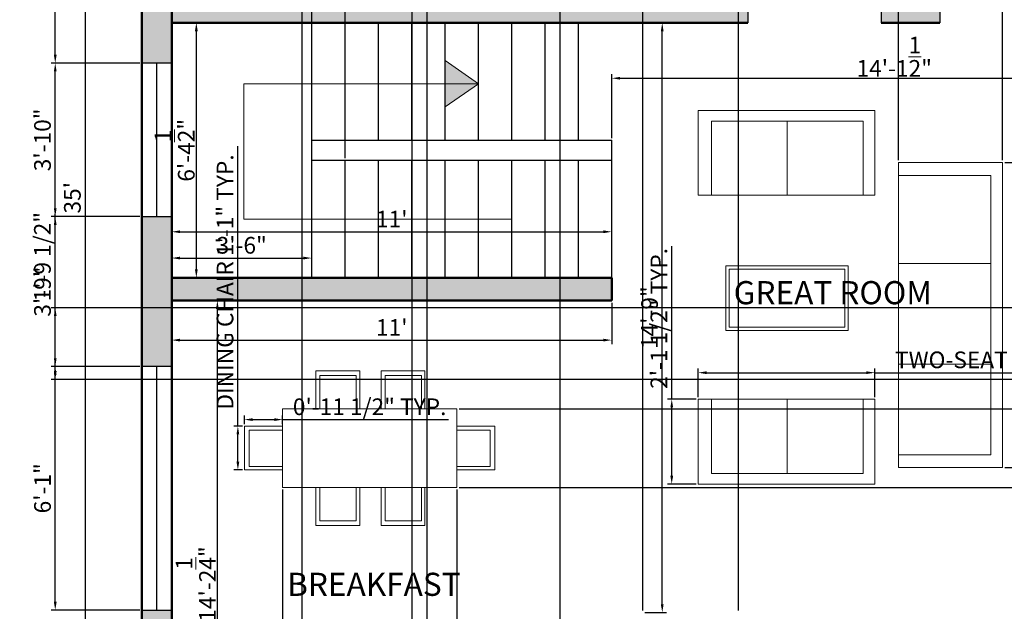
# Model space of a CAD drawing. Units: inches. Extents: x 2168 to 2706, y 2255 to 2760.
# Tile 2 of 4: x 2168 to 2463, y 2389 to 2567. Entities that reach past the tile are written whole.
import ezdxf

# ---------------------------------------------------------------- set-up
doc = ezdxf.new("R2010")
doc.units = ezdxf.units.IN
for name, color, linetype, lineweight in [('A-ANNO-DIMS', 220, 'Continuous', 18), ('A-ANNO-SYMB', 10, 'Continuous', 18), ('A-AREA-IDEN', 220, 'Continuous', 25), ('A-FLOR-STRS', 10, 'Continuous', 25), ('A-WALL-PATT', 140, 'Continuous', 13), ('DOOR', 30, 'Continuous', 25), ('FUR', 112, 'Continuous', 18), ('WALL', 140, 'Continuous', 50), ('WINDOW', 200, 'Continuous', 25)]:
    doc.layers.add(name, color=color, linetype=linetype, lineweight=lineweight)
doc.styles.get("Standard").update_dxf_attribs({"font": 'arial.ttf'})
doc.dimstyles.new('ISO-25', dxfattribs={"dimtxt": 5, "dimasz": 2.5, "dimexe": 1.25, "dimexo": 0.625, "dimtad": 1, "dimlunit": 4, "dimtxsty": 'Standard', "dimcen": 2.5, "dimadec": 0, "dimazin": 0, "dimtfac": 1, "dimtmove": 0, "dimatfit": 3, "dimfxl": 1, "dimarcsym": 0})

# ---------------------------------------------------------------- blocks, each defined once
blk = doc.blocks.new('*U2')
for p, q in [((0, 0), (0, -6)), ((40, 0), (40, -6))]:
    blk.add_line(p, q)
blk.add_lwpolyline([(0, 0), (0, 40), (1.75, 40), (1.75, 0)], close=True)
blk.add_arc((0, 0), 40, 0, 90)
blk = doc.blocks.new('*D20')
at = {"layer": 'A-ANNO-DIMS', "color": 0, "lineweight": -2, "transparency": 16777216}
for p, q in [((2213.72, 2489.97), (2213.72, 2504.39)), ((2216.22, 2503.14), (2343.22, 2503.14)), ((2345.72, 2489.97), (2345.72, 2504.39))]:
    blk.add_line(p, q, dxfattribs=at)
at = {"layer": 'A-ANNO-DIMS', "color": 0, "transparency": 16777216}
for points in [[(2216.22, 2503.56), (2216.22, 2502.73), (2213.72, 2503.14)], [(2343.22, 2503.56), (2343.22, 2502.73), (2345.72, 2503.14)]]:
    blk.add_solid(points, dxfattribs=at)
at = {"layer": 'Defpoints', "color": 0, "transparency": 16777216}
for p in [(2345.72, 2503.14), (2213.72, 2489.35), (2345.72, 2489.35)]:
    blk.add_point(p, dxfattribs=at)
at = {"layer": 'A-ANNO-DIMS', "color": 0, "transparency": 16777216, "insert": (2279.72, 2506.28), "char_height": 5, "attachment_point": 5}
blk.add_mtext("11'", dxfattribs=at)
blk = doc.blocks.new('*D21')
at = {"layer": 'A-ANNO-DIMS', "color": 0, "lineweight": -2, "transparency": 16777216}
for p, q in [((2213.72, 2489.97), (2213.72, 2496.5)), ((2255.72, 2489.97), (2255.72, 2496.5)), ((2216.22, 2495.25), (2253.22, 2495.25))]:
    blk.add_line(p, q, dxfattribs=at)
at = {"layer": 'A-ANNO-DIMS', "color": 0, "transparency": 16777216}
for points in [[(2216.22, 2495.67), (2216.22, 2494.83), (2213.72, 2495.25)], [(2253.22, 2495.67), (2253.22, 2494.83), (2255.72, 2495.25)]]:
    blk.add_solid(points, dxfattribs=at)
at = {"layer": 'Defpoints', "color": 0, "transparency": 16777216}
for p in [(2255.72, 2495.25), (2213.72, 2489.35), (2255.72, 2489.35)]:
    blk.add_point(p, dxfattribs=at)
at = {"layer": 'A-ANNO-DIMS', "color": 0, "transparency": 16777216, "insert": (2234.72, 2498.43), "char_height": 5, "attachment_point": 5}
blk.add_mtext('3\'-6"', dxfattribs=at)
blk = doc.blocks.new('*D22')
at = {"layer": 'A-ANNO-DIMS', "color": 0, "lineweight": -2, "transparency": 16777216}
for p, q in [((2214.35, 2565.85), (2222.35, 2565.85)), ((2221.1, 2491.85), (2221.1, 2563.35)), ((2214.35, 2489.35), (2222.35, 2489.35))]:
    blk.add_line(p, q, dxfattribs=at)
at = {"layer": 'A-ANNO-DIMS', "color": 0, "transparency": 16777216}
for points in [[(2220.68, 2563.35), (2221.52, 2563.35), (2221.1, 2565.85)], [(2220.68, 2491.85), (2221.52, 2491.85), (2221.1, 2489.35)]]:
    blk.add_solid(points, dxfattribs=at)
at = {"layer": 'Defpoints', "color": 0, "transparency": 16777216}
for p in [(2213.72, 2565.85), (2221.1, 2565.85), (2213.72, 2489.35)]:
    blk.add_point(p, dxfattribs=at)
at = {"layer": 'A-ANNO-DIMS', "color": 0, "transparency": 16777216, "insert": (2214.58, 2527.6), "char_height": 5, "attachment_point": 5, "rotation": 90}
blk.add_mtext('6\'-4{\\H1x;\\S1/2;}"', dxfattribs=at)
blk = doc.blocks.new('*D23')
at = {"layer": 'A-ANNO-DIMS', "color": 0, "lineweight": -2, "transparency": 16777216}
for p, q in [((2345.72, 2531.22), (2345.72, 2550.47)), ((2348.22, 2549.22), (2512.72, 2549.22)), ((2515.22, 2531.22), (2515.22, 2550.47))]:
    blk.add_line(p, q, dxfattribs=at)
at = {"layer": 'A-ANNO-DIMS', "color": 0, "transparency": 16777216}
for points in [[(2348.22, 2549.63), (2348.22, 2548.8), (2345.72, 2549.22)], [(2512.72, 2549.63), (2512.72, 2548.8), (2515.22, 2549.22)]]:
    blk.add_solid(points, dxfattribs=at)
at = {"layer": 'Defpoints', "color": 0, "transparency": 16777216}
for p in [(2515.22, 2549.22), (2345.72, 2530.6), (2515.22, 2530.6)]:
    blk.add_point(p, dxfattribs=at)
at = {"layer": 'A-ANNO-DIMS', "color": 0, "transparency": 16777216, "insert": (2430.47, 2555.69), "char_height": 5, "attachment_point": 5}
blk.add_mtext('14\'-1{\\H1x;\\S1/2;}"', dxfattribs=at)
blk = doc.blocks.new('*D24')
at = {"layer": 'A-ANNO-DIMS', "color": 0, "lineweight": -2, "transparency": 16777216}
for p, q in [((2355.67, 2565.85), (2362.12, 2565.85)), ((2360.87, 2391.35), (2360.87, 2563.35)), ((2355.67, 2388.85), (2362.12, 2388.85))]:
    blk.add_line(p, q, dxfattribs=at)
at = {"layer": 'A-ANNO-DIMS', "color": 0, "transparency": 16777216}
for points in [[(2360.45, 2563.35), (2361.28, 2563.35), (2360.87, 2565.85)], [(2360.45, 2391.35), (2361.28, 2391.35), (2360.87, 2388.85)]]:
    blk.add_solid(points, dxfattribs=at)
at = {"layer": 'Defpoints', "color": 0, "transparency": 16777216}
for p in [(2355.04, 2565.85), (2360.87, 2565.85), (2355.04, 2388.85)]:
    blk.add_point(p, dxfattribs=at)
at = {"layer": 'A-ANNO-DIMS', "color": 0, "transparency": 16777216, "insert": (2357.69, 2477.35), "char_height": 5, "attachment_point": 5, "rotation": 90}
blk.add_mtext('14\'-9"', dxfattribs=at)
blk = doc.blocks.new('*D25')
at = {"layer": 'A-ANNO-DIMS', "color": 0, "lineweight": -2, "transparency": 16777216}
for p, q in [((2213.72, 2481.86), (2213.72, 2469.37)), ((2345.72, 2481.86), (2345.72, 2469.37)), ((2216.22, 2470.62), (2343.22, 2470.62))]:
    blk.add_line(p, q, dxfattribs=at)
at = {"layer": 'A-ANNO-DIMS', "color": 0, "transparency": 16777216}
for points in [[(2216.22, 2471.04), (2216.22, 2470.21), (2213.72, 2470.62)], [(2343.22, 2471.04), (2343.22, 2470.21), (2345.72, 2470.62)]]:
    blk.add_solid(points, dxfattribs=at)
at = {"layer": 'Defpoints', "color": 0, "transparency": 16777216}
for p in [(2213.72, 2482.49), (2345.72, 2482.49), (2345.72, 2470.62)]:
    blk.add_point(p, dxfattribs=at)
at = {"layer": 'A-ANNO-DIMS', "color": 0, "transparency": 16777216, "insert": (2279.72, 2473.76), "char_height": 5, "attachment_point": 5}
blk.add_mtext("11'", dxfattribs=at)
blk = doc.blocks.new('*D28')
at = {"layer": 'A-ANNO-DIMS', "color": 0, "lineweight": -2, "transparency": 16777216}
for p, q in [((2214.35, 2482.49), (2228.66, 2482.49)), ((2227.41, 2314.85), (2227.41, 2479.99)), ((2214.35, 2312.35), (2228.66, 2312.35))]:
    blk.add_line(p, q, dxfattribs=at)
at = {"layer": 'A-ANNO-DIMS', "color": 0, "transparency": 16777216}
for points in [[(2227, 2479.99), (2227.83, 2479.99), (2227.41, 2482.49)], [(2227, 2314.85), (2227.83, 2314.85), (2227.41, 2312.35)]]:
    blk.add_solid(points, dxfattribs=at)
at = {"layer": 'Defpoints', "color": 0, "transparency": 16777216}
for p in [(2213.72, 2482.49), (2227.41, 2482.49), (2213.72, 2312.35)]:
    blk.add_point(p, dxfattribs=at)
at = {"layer": 'A-ANNO-DIMS', "color": 0, "transparency": 16777216, "insert": (2220.94, 2397.42), "char_height": 5, "attachment_point": 5, "rotation": 90}
blk.add_mtext('14\'-2{\\H1x;\\S1/4;}"', dxfattribs=at)
blk = doc.blocks.new('*D30')
at = {"layer": 'A-ANNO-DIMS', "color": 0, "lineweight": -2, "transparency": 16777216}
for p, q in [((2204.1, 2723.35), (2186.49, 2723.35)), ((2187.74, 2720.85), (2187.74, 2305.85)), ((2204.1, 2303.35), (2186.49, 2303.35))]:
    blk.add_line(p, q, dxfattribs=at)
at = {"layer": 'A-ANNO-DIMS', "color": 0, "transparency": 16777216}
for points in [[(2187.33, 2720.85), (2188.16, 2720.85), (2187.74, 2723.35)], [(2187.33, 2305.85), (2188.16, 2305.85), (2187.74, 2303.35)]]:
    blk.add_solid(points, dxfattribs=at)
at = {"layer": 'Defpoints', "color": 0, "transparency": 16777216}
for p in [(2204.72, 2723.35), (2187.74, 2303.35), (2204.72, 2303.35)]:
    blk.add_point(p, dxfattribs=at)
at = {"layer": 'A-ANNO-DIMS', "color": 0, "transparency": 16777216, "insert": (2184.56, 2513.35), "char_height": 5, "attachment_point": 5, "rotation": 90}
blk.add_mtext("35'", dxfattribs=at)
blk = doc.blocks.new('CHAIR-DINING')
for p, q in [((-11.42, -6.49), (-11.42, 6.66)), ((-11.42, 6.66), (0, 6.66)), ((0, -6.49), (-11.42, -6.49))]:
    blk.add_line(p, q)
blk.add_lwpolyline([(0, 5.44), (-10.02, 5.44), (-10.02, -5.44), (0, -5.44)], close=True)
blk = doc.blocks.new('SOFA-TWO-SEAT')
for p, q in [((3.96, 25.48), (0, 25.48)), ((0, 25.48), (0, 0)), ((26.73, 25.48), (26.73, 3.2)), ((52.95, 25.48), (48.19, 25.48)), ((52.95, 0), (52.95, 25.48)), ((0, 0), (52.95, 0))]:
    blk.add_line(p, q)
blk.add_lwpolyline([(49.5, 3.2), (3.96, 3.2), (3.96, 25.48), (49.5, 25.48)], close=True)
blk = doc.blocks.new('*D38')
at = {"layer": 'A-ANNO-DIMS', "color": 0, "lineweight": -2, "transparency": 16777216}
for p, q in [((2233.56, 2444.79), (2233.56, 2528.83)), ((2234.91, 2444.79), (2232.31, 2444.79)), ((2233.56, 2434.14), (2233.56, 2442.29)), ((2234.91, 2431.64), (2232.31, 2431.64))]:
    blk.add_line(p, q, dxfattribs=at)
at = {"layer": 'A-ANNO-DIMS', "color": 0, "transparency": 16777216}
for points in [[(2233.14, 2442.29), (2233.98, 2442.29), (2233.56, 2444.79)], [(2233.14, 2434.14), (2233.98, 2434.14), (2233.56, 2431.64)]]:
    blk.add_solid(points, dxfattribs=at)
at = {"layer": 'Defpoints', "color": 0, "transparency": 16777216}
for p in [(2233.56, 2444.79), (2235.53, 2444.79), (2235.53, 2431.64)]:
    blk.add_point(p, dxfattribs=at)
at = {"layer": 'A-ANNO-DIMS', "color": 0, "transparency": 16777216, "insert": (2230.35, 2488.06), "char_height": 5, "attachment_point": 5, "rotation": 90}
blk.add_mtext('DINING CHAIR 1\'-1" TYP.', dxfattribs=at)
blk = doc.blocks.new('*D39')
at = {"layer": 'A-ANNO-DIMS', "color": 0, "lineweight": -2, "transparency": 16777216}
for p, q in [((2235.53, 2445.41), (2235.53, 2448.01)), ((2238.03, 2446.76), (2244.46, 2446.76)), ((2246.96, 2445.41), (2246.96, 2448.01)), ((2246.96, 2446.76), (2296.72, 2446.76))]:
    blk.add_line(p, q, dxfattribs=at)
at = {"layer": 'A-ANNO-DIMS', "color": 0, "transparency": 16777216}
for points in [[(2238.03, 2447.18), (2238.03, 2446.34), (2235.53, 2446.76)], [(2244.46, 2447.18), (2244.46, 2446.34), (2246.96, 2446.76)]]:
    blk.add_solid(points, dxfattribs=at)
at = {"layer": 'Defpoints', "color": 0, "transparency": 16777216}
for p in [(2246.96, 2446.76), (2235.53, 2444.79), (2246.96, 2444.79)]:
    blk.add_point(p, dxfattribs=at)
at = {"layer": 'A-ANNO-DIMS', "color": 0, "transparency": 16777216, "insert": (2273.09, 2449.97), "char_height": 5, "attachment_point": 5}
blk.add_mtext('0\'-11 1/2" TYP.', dxfattribs=at)
blk = doc.blocks.new('*D40')
at = {"layer": 'A-ANNO-DIMS', "color": 0, "lineweight": -2, "transparency": 16777216}
for p, q in [((2371.67, 2453.52), (2371.67, 2462.09)), ((2374.17, 2460.84), (2422.11, 2460.84)), ((2424.61, 2453.52), (2424.61, 2462.09)), ((2424.61, 2460.84), (2518.73, 2460.84))]:
    blk.add_line(p, q, dxfattribs=at)
at = {"layer": 'A-ANNO-DIMS', "color": 0, "transparency": 16777216}
for points in [[(2374.17, 2461.26), (2374.17, 2460.43), (2371.67, 2460.84)], [(2422.11, 2461.26), (2422.11, 2460.43), (2424.61, 2460.84)]]:
    blk.add_solid(points, dxfattribs=at)
at = {"layer": 'Defpoints', "color": 0, "transparency": 16777216}
for p in [(2424.61, 2460.84), (2371.67, 2452.9), (2424.61, 2452.9)]:
    blk.add_point(p, dxfattribs=at)
at = {"layer": 'A-ANNO-DIMS', "color": 0, "transparency": 16777216, "insert": (2472.92, 2464.05), "char_height": 5, "attachment_point": 5}
blk.add_mtext('TWO-SEAT SOFA 4\'-5" TYP.', dxfattribs=at)
blk = doc.blocks.new('*D41')
at = {"layer": 'A-ANNO-DIMS', "color": 0, "lineweight": -2, "transparency": 16777216}
for p, q in [((2363.72, 2452.9), (2363.72, 2498.86)), ((2371.04, 2452.9), (2362.47, 2452.9)), ((2363.72, 2429.92), (2363.72, 2450.4)), ((2371.04, 2427.42), (2362.47, 2427.42))]:
    blk.add_line(p, q, dxfattribs=at)
at = {"layer": 'A-ANNO-DIMS', "color": 0, "transparency": 16777216}
for points in [[(2363.31, 2450.4), (2364.14, 2450.4), (2363.72, 2452.9)], [(2363.31, 2429.92), (2364.14, 2429.92), (2363.72, 2427.42)]]:
    blk.add_solid(points, dxfattribs=at)
at = {"layer": 'Defpoints', "color": 0, "transparency": 16777216}
for p in [(2363.72, 2452.9), (2371.67, 2452.9), (2371.67, 2427.42)]:
    blk.add_point(p, dxfattribs=at)
at = {"layer": 'A-ANNO-DIMS', "color": 0, "transparency": 16777216, "insert": (2360.51, 2477.13), "char_height": 5, "attachment_point": 5, "rotation": 90}
blk.add_mtext('2\'-1 1/2" TYP.', dxfattribs=at)
blk = doc.blocks.new('*D49')
at = {"layer": 'A-ANNO-DIMS', "color": 0, "lineweight": -2, "transparency": 16777216}
for p, q in [((2355.04, 2389.47), (2355.04, 2750.55)), ((2383.78, 2389.47), (2383.78, 2750.55)), ((2357.54, 2749.3), (2381.28, 2749.3))]:
    blk.add_line(p, q, dxfattribs=at)
at = {"layer": 'A-ANNO-DIMS', "color": 0, "transparency": 16777216}
for points in [[(2357.54, 2749.71), (2357.54, 2748.88), (2355.04, 2749.3)], [(2381.28, 2749.71), (2381.28, 2748.88), (2383.78, 2749.3)]]:
    blk.add_solid(points, dxfattribs=at)
at = {"layer": 'Defpoints', "color": 0, "transparency": 16777216}
for p in [(2383.78, 2749.3), (2355.04, 2388.85), (2383.78, 2388.85)]:
    blk.add_point(p, dxfattribs=at)
at = {"layer": 'A-ANNO-DIMS', "color": 0, "transparency": 16777216, "insert": (2369.41, 2752.51), "char_height": 5, "attachment_point": 5}
blk.add_mtext('2\'-4 1/2"', dxfattribs=at)
blk = doc.blocks.new('*D51')
at = {"layer": 'A-ANNO-DIMS', "color": 0, "lineweight": -2, "transparency": 16777216}
for p, q in [((2178.77, 2480.31), (2178.77, 2508.53)), ((2538.6, 2480.31), (2177.52, 2480.31)), ((2178.77, 2461.31), (2178.77, 2477.81)), ((2538.6, 2458.81), (2177.52, 2458.81))]:
    blk.add_line(p, q, dxfattribs=at)
at = {"layer": 'A-ANNO-DIMS', "color": 0, "transparency": 16777216}
for points in [[(2178.36, 2477.81), (2179.19, 2477.81), (2178.77, 2480.31)], [(2178.36, 2461.31), (2179.19, 2461.31), (2178.77, 2458.81)]]:
    blk.add_solid(points, dxfattribs=at)
at = {"layer": 'Defpoints', "color": 0, "transparency": 16777216}
for p in [(2178.77, 2480.31), (2539.22, 2480.31), (2539.22, 2458.81)]:
    blk.add_point(p, dxfattribs=at)
at = {"layer": 'A-ANNO-DIMS', "color": 0, "transparency": 16777216, "insert": (2175.56, 2495.67), "char_height": 5, "attachment_point": 5, "rotation": 90}
blk.add_mtext('1\'-9 1/2"', dxfattribs=at)
blk = doc.blocks.new('*D52')
at = {"layer": 'A-ANNO-DIMS', "color": 0, "lineweight": -2, "transparency": 16777216}
for p, q in [((2463.6, 2523.98), (2702.92, 2523.98)), ((2701.67, 2434.92), (2701.67, 2521.48)), ((2463.6, 2432.42), (2702.92, 2432.42))]:
    blk.add_line(p, q, dxfattribs=at)
at = {"layer": 'A-ANNO-DIMS', "color": 0, "transparency": 16777216}
for points in [[(2701.26, 2521.48), (2702.09, 2521.48), (2701.67, 2523.98)], [(2701.26, 2434.92), (2702.09, 2434.92), (2701.67, 2432.42)]]:
    blk.add_solid(points, dxfattribs=at)
at = {"layer": 'Defpoints', "color": 0, "transparency": 16777216}
for p in [(2462.98, 2523.98), (2701.67, 2523.98), (2462.98, 2432.42)]:
    blk.add_point(p, dxfattribs=at)
at = {"layer": 'A-ANNO-DIMS', "color": 0, "transparency": 16777216, "insert": (2698.46, 2478.2), "char_height": 5, "attachment_point": 5, "rotation": 90}
blk.add_mtext('7\'-7 1/2"', dxfattribs=at)
blk = doc.blocks.new('*D53')
at = {"layer": 'A-ANNO-DIMS', "color": 0, "lineweight": -2, "transparency": 16777216}
for p, q in [((2431.71, 2524.6), (2431.71, 2750.55)), ((2462.98, 2524.6), (2462.98, 2750.55)), ((2434.21, 2749.3), (2460.48, 2749.3))]:
    blk.add_line(p, q, dxfattribs=at)
at = {"layer": 'A-ANNO-DIMS', "color": 0, "transparency": 16777216}
for points in [[(2434.21, 2749.71), (2434.21, 2748.88), (2431.71, 2749.3)], [(2460.48, 2749.71), (2460.48, 2748.88), (2462.98, 2749.3)]]:
    blk.add_solid(points, dxfattribs=at)
at = {"layer": 'Defpoints', "color": 0, "transparency": 16777216}
for p in [(2462.98, 2749.3), (2431.71, 2523.98), (2462.98, 2523.98)]:
    blk.add_point(p, dxfattribs=at)
at = {"layer": 'A-ANNO-DIMS', "color": 0, "transparency": 16777216, "insert": (2447.34, 2752.51), "char_height": 5, "attachment_point": 5}
blk.add_mtext('2\'-7 1/2"', dxfattribs=at)
blk = doc.blocks.new('*D54')
at = {"layer": 'A-ANNO-DIMS', "color": 0, "lineweight": -2, "transparency": 16777216}
for p, q in [((2246.96, 2425.79), (2246.96, 2276.15)), ((2299.27, 2425.79), (2299.27, 2276.15)), ((2249.46, 2277.4), (2296.77, 2277.4))]:
    blk.add_line(p, q, dxfattribs=at)
at = {"layer": 'A-ANNO-DIMS', "color": 0, "transparency": 16777216}
for points in [[(2249.46, 2277.81), (2249.46, 2276.98), (2246.96, 2277.4)], [(2296.77, 2277.81), (2296.77, 2276.98), (2299.27, 2277.4)]]:
    blk.add_solid(points, dxfattribs=at)
at = {"layer": 'Defpoints', "color": 0, "transparency": 16777216}
for p in [(2246.96, 2426.42), (2299.27, 2426.42), (2299.27, 2277.4)]:
    blk.add_point(p, dxfattribs=at)
at = {"layer": 'A-ANNO-DIMS', "color": 0, "transparency": 16777216, "insert": (2273.11, 2280.61), "char_height": 5, "attachment_point": 5}
blk.add_mtext('4\'-4 1/2"', dxfattribs=at)
blk = doc.blocks.new('*D55')
at = {"layer": 'A-ANNO-DIMS', "color": 0, "lineweight": -2, "transparency": 16777216}
for p, q in [((2299.9, 2450), (2702.92, 2450)), ((2701.67, 2447.5), (2701.67, 2428.92)), ((2299.9, 2426.42), (2702.92, 2426.42)), ((2701.67, 2426.42), (2701.67, 2394.31))]:
    blk.add_line(p, q, dxfattribs=at)
at = {"layer": 'A-ANNO-DIMS', "color": 0, "transparency": 16777216}
for points in [[(2701.26, 2447.5), (2702.09, 2447.5), (2701.67, 2450)], [(2701.26, 2428.92), (2702.09, 2428.92), (2701.67, 2426.42)]]:
    blk.add_solid(points, dxfattribs=at)
at = {"layer": 'Defpoints', "color": 0, "transparency": 16777216}
for p in [(2299.27, 2450), (2299.27, 2426.42), (2701.67, 2426.42)]:
    blk.add_point(p, dxfattribs=at)
at = {"layer": 'A-ANNO-DIMS', "color": 0, "transparency": 16777216, "insert": (2698.46, 2409.11), "char_height": 5, "attachment_point": 5, "rotation": 90}
blk.add_mtext('1\'-11 1/2"', dxfattribs=at)
blk = doc.blocks.new('*D64')
at = {"layer": 'A-ANNO-DIMS', "color": 0, "lineweight": -2, "transparency": 16777216}
for p, q in [((2290.22, 2713.72), (2290.22, 2276.15)), ((2330.12, 2713.72), (2330.12, 2276.15)), ((2292.72, 2277.4), (2327.62, 2277.4))]:
    blk.add_line(p, q, dxfattribs=at)
at = {"layer": 'A-ANNO-DIMS', "color": 0, "transparency": 16777216}
for points in [[(2292.72, 2277.81), (2292.72, 2276.98), (2290.22, 2277.4)], [(2327.62, 2277.81), (2327.62, 2276.98), (2330.12, 2277.4)]]:
    blk.add_solid(points, dxfattribs=at)
at = {"layer": 'Defpoints', "color": 0, "transparency": 16777216}
for p in [(2290.22, 2714.35), (2330.12, 2714.35), (2330.12, 2277.4)]:
    blk.add_point(p, dxfattribs=at)
at = {"layer": 'A-ANNO-DIMS', "color": 0, "transparency": 16777216, "insert": (2310.17, 2280.58), "char_height": 5, "attachment_point": 5}
blk.add_mtext('3\'-4"', dxfattribs=at)
blk = doc.blocks.new('*D66')
at = {"layer": 'A-ANNO-DIMS', "color": 0, "lineweight": -2, "transparency": 16777216}
for p, q in [((2204.1, 2462.7), (2177.52, 2462.7)), ((2178.77, 2392.09), (2178.77, 2460.2)), ((2204.1, 2389.59), (2177.52, 2389.59))]:
    blk.add_line(p, q, dxfattribs=at)
at = {"layer": 'A-ANNO-DIMS', "color": 0, "transparency": 16777216}
for points in [[(2178.36, 2460.2), (2179.19, 2460.2), (2178.77, 2462.7)], [(2178.36, 2392.09), (2179.19, 2392.09), (2178.77, 2389.59)]]:
    blk.add_solid(points, dxfattribs=at)
at = {"layer": 'Defpoints', "color": 0, "transparency": 16777216}
for p in [(2178.77, 2462.7), (2204.72, 2462.7), (2204.72, 2389.59)]:
    blk.add_point(p, dxfattribs=at)
at = {"layer": 'A-ANNO-DIMS', "color": 0, "transparency": 16777216, "insert": (2175.6, 2426.14), "char_height": 5, "attachment_point": 5, "rotation": 90}
blk.add_mtext('6\'-1"', dxfattribs=at)
blk = doc.blocks.new('*D67')
at = {"layer": 'A-ANNO-DIMS', "color": 0, "lineweight": -2, "transparency": 16777216}
for p, q in [((2204.1, 2553.76), (2177.52, 2553.76)), ((2178.77, 2510.18), (2178.77, 2551.26)), ((2204.1, 2507.68), (2177.52, 2507.68))]:
    blk.add_line(p, q, dxfattribs=at)
at = {"layer": 'A-ANNO-DIMS', "color": 0, "transparency": 16777216}
for points in [[(2178.36, 2551.26), (2179.19, 2551.26), (2178.77, 2553.76)], [(2178.36, 2510.18), (2179.19, 2510.18), (2178.77, 2507.68)]]:
    blk.add_solid(points, dxfattribs=at)
at = {"layer": 'Defpoints', "color": 0, "transparency": 16777216}
for p in [(2178.77, 2553.76), (2204.72, 2553.76), (2204.72, 2507.68)]:
    blk.add_point(p, dxfattribs=at)
at = {"layer": 'A-ANNO-DIMS', "color": 0, "transparency": 16777216, "insert": (2175.59, 2530.72), "char_height": 5, "attachment_point": 5, "rotation": 90}
blk.add_mtext('3\'-10"', dxfattribs=at)
blk = doc.blocks.new('*D70')
at = {"layer": 'A-ANNO-DIMS', "color": 0, "lineweight": -2, "transparency": 16777216}
for p, q in [((2204.1, 2507.68), (2177.52, 2507.68)), ((2178.77, 2465.2), (2178.77, 2505.18)), ((2204.1, 2462.7), (2177.52, 2462.7))]:
    blk.add_line(p, q, dxfattribs=at)
at = {"layer": 'A-ANNO-DIMS', "color": 0, "transparency": 16777216}
for points in [[(2178.36, 2505.18), (2179.19, 2505.18), (2178.77, 2507.68)], [(2178.36, 2465.2), (2179.19, 2465.2), (2178.77, 2462.7)]]:
    blk.add_solid(points, dxfattribs=at)
at = {"layer": 'Defpoints', "color": 0, "transparency": 16777216}
for p in [(2178.77, 2507.68), (2204.72, 2507.68), (2204.72, 2462.7)]:
    blk.add_point(p, dxfattribs=at)
at = {"layer": 'A-ANNO-DIMS', "color": 0, "transparency": 16777216, "insert": (2175.59, 2485.19), "char_height": 5, "attachment_point": 5, "rotation": 90}
blk.add_mtext('3\'-9"', dxfattribs=at)
blk = doc.blocks.new('*D71')
at = {"layer": 'A-ANNO-DIMS', "color": 0, "lineweight": -2, "transparency": 16777216}
for p, q in [((2204.1, 2613.73), (2177.52, 2613.73)), ((2178.77, 2556.26), (2178.77, 2611.23)), ((2204.1, 2553.76), (2177.52, 2553.76))]:
    blk.add_line(p, q, dxfattribs=at)
at = {"layer": 'A-ANNO-DIMS', "color": 0, "transparency": 16777216}
for points in [[(2178.36, 2611.23), (2179.19, 2611.23), (2178.77, 2613.73)], [(2178.36, 2556.26), (2179.19, 2556.26), (2178.77, 2553.76)]]:
    blk.add_solid(points, dxfattribs=at)
at = {"layer": 'Defpoints', "color": 0, "transparency": 16777216}
for p in [(2178.77, 2613.73), (2204.72, 2613.73), (2204.72, 2553.76)]:
    blk.add_point(p, dxfattribs=at)
at = {"layer": 'A-ANNO-DIMS', "color": 0, "transparency": 16777216, "insert": (2175.6, 2583.75), "char_height": 5, "attachment_point": 5, "rotation": 90}
blk.add_mtext('5\'-0"', dxfattribs=at)
blk = doc.blocks.new('*D74')
at = {"layer": 'A-ANNO-DIMS', "color": 0, "lineweight": -2, "transparency": 16777216}
for p, q in [((2255.72, 2525.22), (2255.72, 2750.55)), ((2265.72, 2525.22), (2265.72, 2750.55)), ((2258.22, 2749.3), (2263.22, 2749.3)), ((2265.72, 2749.3), (2286.65, 2749.3))]:
    blk.add_line(p, q, dxfattribs=at)
at = {"layer": 'A-ANNO-DIMS', "color": 0, "transparency": 16777216}
for points in [[(2258.22, 2749.71), (2258.22, 2748.88), (2255.72, 2749.3)], [(2263.22, 2749.71), (2263.22, 2748.88), (2265.72, 2749.3)]]:
    blk.add_solid(points, dxfattribs=at)
at = {"layer": 'Defpoints', "color": 0, "transparency": 16777216}
for p in [(2265.72, 2749.3), (2255.72, 2524.6), (2265.72, 2524.6)]:
    blk.add_point(p, dxfattribs=at)
at = {"layer": 'A-ANNO-DIMS', "color": 0, "transparency": 16777216, "insert": (2277.44, 2752.47), "char_height": 5, "attachment_point": 5}
blk.add_mtext('0\'-10"', dxfattribs=at)
blk = doc.blocks.new('*D76')
at = {"layer": 'A-ANNO-DIMS', "color": 0, "lineweight": -2, "transparency": 16777216}
for p, q in [((2252.72, 2623.46), (2252.72, 2276.15)), ((2285.72, 2612.95), (2285.72, 2276.15)), ((2255.22, 2277.4), (2283.22, 2277.4))]:
    blk.add_line(p, q, dxfattribs=at)
at = {"layer": 'A-ANNO-DIMS', "color": 0, "transparency": 16777216}
for points in [[(2255.22, 2277.81), (2255.22, 2276.98), (2252.72, 2277.4)], [(2283.22, 2277.81), (2283.22, 2276.98), (2285.72, 2277.4)]]:
    blk.add_solid(points, dxfattribs=at)
at = {"layer": 'Defpoints', "color": 0, "transparency": 16777216}
for p in [(2252.72, 2624.08), (2285.72, 2613.58), (2285.72, 2277.4)]:
    blk.add_point(p, dxfattribs=at)
at = {"layer": 'A-ANNO-DIMS', "color": 0, "transparency": 16777216, "insert": (2269.22, 2280.57), "char_height": 5, "attachment_point": 5}
blk.add_mtext('2\'-9"', dxfattribs=at)

msp = doc.modelspace()

# ---------------------------------------------------------------- hatches: boundary and pattern name
at = {"layer": 'A-ANNO-SYMB'}
h = msp.add_hatch(color=256, dxfattribs=at)
h.dxf.hatch_style = 1
h.paths.add_polyline_path([(2305.724, 2547.588), (2295.724, 2547.588), (2295.724, 2540.636)])
h.paths.add_polyline_path([(2295.724, 2554.541), (2295.724, 2547.588), (2305.724, 2547.588)])
at = {"layer": 'A-WALL-PATT'}
h = msp.add_hatch(color=256, dxfattribs=at)
h.dxf.hatch_style = 1
h.paths.add_polyline_path([(2330.12, 2723.347), (2204.724, 2723.347), (2204.724, 2662.147), (2213.724, 2662.147), (2213.724, 2714.347), (2285.724, 2714.347), (2330.12, 2714.347)])
h.paths.add_polyline_path([(2496.542, 2723.347), (2396.128, 2723.347), (2396.128, 2714.347), (2434.224, 2714.347), (2496.542, 2714.347)])
h.paths.add_polyline_path([(2624.724, 2723.347), (2562.55, 2723.347), (2562.55, 2714.347), (2615.724, 2714.347), (2615.724, 2545.448), (2624.724, 2545.448)])
h.paths.add_polyline_path([(2438.724, 2714.347), (2434.224, 2714.347), (2434.224, 2570.347), (2426.591, 2570.347), (2426.591, 2565.847), (2438.724, 2565.847), (2444.149, 2565.847), (2444.149, 2570.347), (2438.724, 2570.347)])
h.paths.add_polyline_path([(2290.224, 2668.023), (2285.724, 2668.023), (2285.724, 2570.347), (2213.724, 2570.347), (2213.724, 2565.847), (2290.224, 2565.847), (2386.591, 2565.847), (2386.591, 2570.347), (2290.224, 2570.347)])
h.paths.add_polyline_path([(2514.678, 2570.347), (2514.678, 2630.11), (2560.439, 2630.11), (2560.439, 2570.347)], flags=16)
h.paths.add_polyline_path([(2517.528, 2574.595), (2517.528, 2583.399), (2536.063, 2583.399), (2536.063, 2574.595)], flags=0)
h.paths.add_polyline_path([(2523.909, 2586.89), (2514.678, 2597.212), (2518.822, 2600.918)], flags=0)
h.paths.add_polyline_path([(2538.189, 2574.595), (2538.189, 2583.399), (2556.724, 2583.399), (2556.724, 2574.595)], flags=0)
h.paths.add_polyline_path([(2560.439, 2630.11), (2560.439, 2570.347), (2514.678, 2570.347), (2514.678, 2630.11)])
h.paths.add_polyline_path([(2213.724, 2389.588), (2204.724, 2389.588), (2204.724, 2303.347), (2229.06, 2303.347), (2229.06, 2312.347), (2213.724, 2312.347)])
h.paths.add_polyline_path([(2213.724, 2507.677), (2204.724, 2507.677), (2204.724, 2462.696), (2213.724, 2462.696)])
h.paths.add_polyline_path([(2204.724, 2553.759), (2213.724, 2553.759), (2213.724, 2613.731), (2204.724, 2613.731)])
h = msp.add_hatch(color=256, dxfattribs=at)
h.dxf.hatch_style = 1
h.paths.add_polyline_path([(2345.724, 2489.347), (2213.724, 2489.347), (2213.724, 2482.487), (2345.724, 2482.487)])

# ---------------------------------------------------------------- linework, layer by layer
at = {"layer": 'A-ANNO-SYMB'}
for p, q in [((2305.724, 2547.588), (2295.724, 2554.541)), ((2235.327, 2506.972), (2235.327, 2547.588)), ((2235.327, 2547.588), (2305.724, 2547.588)), ((2305.724, 2547.588), (2295.724, 2540.636)), ((2315.724, 2506.972), (2235.327, 2506.972))]:
    msp.add_line(p, q, dxfattribs=at)
at = {"layer": 'A-FLOR-STRS'}
for p, q in [((2255.724, 2489.347), (2255.724, 2565.847)), ((2265.724, 2530.597), (2265.724, 2565.847)), ((2275.724, 2530.597), (2275.724, 2565.847)), ((2285.724, 2530.597), (2285.724, 2565.847)), ((2295.724, 2530.597), (2295.724, 2565.847)), ((2305.724, 2530.597), (2305.724, 2565.847)), ((2315.724, 2530.597), (2315.724, 2565.847)), ((2325.724, 2530.597), (2325.724, 2565.847)), ((2335.724, 2530.597), (2335.724, 2565.847)), ((2255.724, 2530.597), (2345.724, 2530.597)), ((2345.724, 2489.347), (2345.724, 2530.597)), ((2255.724, 2524.597), (2345.724, 2524.597)), ((2265.724, 2489.347), (2265.724, 2524.597)), ((2275.724, 2489.347), (2275.724, 2524.597)), ((2285.724, 2489.347), (2285.724, 2524.597)), ((2295.724, 2489.347), (2295.724, 2524.597)), ((2305.724, 2489.347), (2305.724, 2524.597)), ((2315.724, 2489.347), (2315.724, 2524.597)), ((2325.724, 2489.347), (2325.724, 2524.597)), ((2335.724, 2489.347), (2335.724, 2524.597)), ((2213.724, 2489.347), (2255.724, 2489.347))]:
    msp.add_line(p, q, dxfattribs=at)
at = {"layer": 'FUR'}
for p, q in [((2431.708, 2520.06), (2459.421, 2520.06)), ((2459.421, 2436.23), (2459.421, 2520.06)), ((2459.421, 2493.599), (2431.708, 2493.599)), ((2459.421, 2463.4), (2431.708, 2463.4)), ((2431.708, 2432.42), (2431.708, 2439.235)), ((2462.979, 2436.23), (2462.979, 2432.42)), ((2462.979, 2432.42), (2431.708, 2432.42))]:
    msp.add_line(p, q, dxfattribs=at)
msp.add_lwpolyline([(2462.979, 2436.23), (2462.979, 2523.979), (2431.708, 2523.979), (2431.708, 2436.23), (2459.421, 2436.23)], dxfattribs=at)
for points in [[(2379.936, 2492.915), (2416.679, 2492.915), (2416.679, 2473.48), (2379.936, 2473.48)], [(2380.936, 2491.915), (2415.679, 2491.915), (2415.679, 2474.48), (2380.936, 2474.48)], [(2246.955, 2449.996), (2299.272, 2449.996), (2299.272, 2426.417), (2246.955, 2426.417)]]:
    msp.add_lwpolyline(points, close=True, dxfattribs=at)
at = {"layer": 'WALL'}
for p, q in [((2204.724, 2303.347), (2204.724, 2723.347)), ((2290.224, 2565.847), (2213.724, 2565.847)), ((2386.591, 2565.847), (2290.224, 2565.847)), ((2438.724, 2565.847), (2426.591, 2565.847)), ((2438.724, 2565.847), (2444.149, 2565.847)), ((2345.724, 2489.347), (2213.724, 2489.347)), ((2345.724, 2489.347), (2345.724, 2482.487)), ((2213.724, 2482.487), (2213.724, 2482.487)), ((2213.724, 2482.487), (2345.724, 2482.487))]:
    msp.add_line(p, q, dxfattribs=at)
for points in [[(2572.054, 2303.347), (2204.724, 2303.347), (2204.724, 2723.347), (2624.724, 2723.347), (2624.724, 2303.347), (2612.054, 2303.347)], [(2572.166, 2312.347), (2213.724, 2312.347), (2213.724, 2714.347), (2615.724, 2714.347), (2615.724, 2312.347), (2610.304, 2312.347)]]:
    msp.add_lwpolyline(points, dxfattribs=at)
at = {"layer": 'WINDOW'}
for p, q in [((2209.224, 2507.677), (2209.224, 2553.759)), ((2209.224, 2389.588), (2209.224, 2462.696))]:
    msp.add_line(p, q, dxfattribs=at)
for points in [[(2204.724, 2507.677), (2213.724, 2507.677), (2213.724, 2553.759), (2204.724, 2553.759)], [(2213.724, 2462.696), (2204.724, 2462.696), (2204.724, 2389.588), (2213.724, 2389.588)]]:
    msp.add_lwpolyline(points, close=True, dxfattribs=at)

# ---------------------------------------------------------------- block references
at = {"layer": 'DOOR', "xscale": -1}
msp.add_blockref('*U2', (2426.591, 2571.847), dxfattribs=at)
at = {"layer": 'DOOR'}
msp.add_blockref('*U2', (2444.149, 2571.847), dxfattribs=at)
at = {"layer": 'FUR', "extrusion": (0, 0, -1), "zscale": -1}
for name, p, rotation in [('SOFA-TWO-SEAT', (-2371.666, 2539.567), 180), ('CHAIR-DINING', (-2263.627, 2449.996), 270.0000000000055), ('CHAIR-DINING', (-2283.207, 2449.996), 270.0000000000055)]:
    msp.add_blockref(name, p, dxfattribs=dict(at, rotation=rotation))
at = {"layer": 'FUR'}
for name, p in [('SOFA-TWO-SEAT', (2371.666, 2427.422)), ('CHAIR-DINING', (2246.955, 2438.131))]:
    msp.add_blockref(name, p, dxfattribs=at)
at = {"layer": 'FUR', "extrusion": (0, 0, -1), "zscale": -1}
msp.add_blockref('CHAIR-DINING', (-2299.272, 2438.131), dxfattribs=at)
at = {"layer": 'FUR', "rotation": 90.00000000000333}
for p in [(2263.627, 2426.417), (2283.207, 2426.417)]:
    msp.add_blockref('CHAIR-DINING', p, dxfattribs=at)

# ---------------------------------------------------------------- texts
at = {"layer": 'A-AREA-IDEN', "char_height": 6.9506, "attachment_point": 1}
for s, heights, insert in [('GREAT ROOM', [6.951], (2382.296, 2488.336)), ('BREAKFAST', [0], (2248.329, 2400.8))]:
    msp.add_mtext_dynamic_manual_height_columns(s, width=121.01281, gutter_width=34.753, heights=heights, dxfattribs=dict(at, insert=insert))

# ---------------------------------------------------------------- dimensions: what is measured, and where the dimension line sits
at = {"layer": 'A-ANNO-DIMS'}
for base, p1, p2, override, picture, middle in [((2383.783, 2749.297), (2355.045, 2388.847), (2383.783, 2388.847), {"dimdec": 1, "dimlfac": 1, "dimrnd": 0, "dimzin": 1, "dimdsep": 46, "dimlunit": 4, "dimfrac": 2}, '*D49', (2369.414, 2752.507)), ((2462.979, 2749.297), (2431.708, 2523.979), (2462.979, 2523.979), {"dimdec": 1, "dimlfac": 1, "dimrnd": 0, "dimzin": 1, "dimdsep": 46, "dimlunit": 4, "dimfrac": 2}, '*D53', (2447.344, 2752.507)), ((2265.724, 2749.297), (2255.724, 2524.597), (2265.724, 2524.597), {"dimdec": 1, "dimlfac": 1, "dimrnd": 0, "dimzin": 1, "dimdsep": 46, "dimlunit": 4, "dimfrac": 2}, '*D74', (2277.437, 2752.475)), ((2330.12, 2277.397), (2290.224, 2714.347), (2330.12, 2714.347), {"dimdec": 1, "dimlfac": 1, "dimrnd": 0, "dimzin": 1, "dimdsep": 46, "dimlunit": 4, "dimfrac": 2}, '*D64', (2310.172, 2280.577)), ((2285.724, 2277.397), (2252.724, 2624.08), (2285.724, 2613.58), {"dimdec": 1, "dimlfac": 1, "dimrnd": 0, "dimzin": 1, "dimdsep": 46, "dimlunit": 4, "dimfrac": 2}, '*D76', (2269.224, 2280.575)), ((2515.224, 2549.215), (2345.724, 2530.597), (2515.224, 2530.597), {"dimclrd": 0, "dimclre": 0, "dimclrt": 0}, '*D23', (2430.474, 2555.694)), ((2345.724, 2503.145), (2213.724, 2489.347), (2345.724, 2489.347), {"dimclrd": 0, "dimclre": 0, "dimclrt": 0}, '*D20', (2279.724, 2506.28)), ((2255.724, 2495.251), (2213.724, 2489.347), (2255.724, 2489.347), {"dimclrd": 0, "dimclre": 0, "dimclrt": 0}, '*D21', (2234.724, 2498.431)), ((2345.724, 2470.622), (2213.724, 2482.487), (2345.724, 2482.487), {"dimclrd": 0, "dimclre": 0, "dimclrt": 0}, '*D25', (2279.724, 2473.757)), ((2299.272, 2277.397), (2246.955, 2426.417), (2299.272, 2426.417), {"dimdec": 1, "dimlfac": 1, "dimrnd": 0, "dimzin": 1, "dimdsep": 46, "dimlunit": 4, "dimfrac": 2}, '*D54', (2273.114, 2280.607))]:
    dim = msp.add_linear_dim(base=base, p1=p1, p2=p2, dimstyle='ISO-25', override=override, dxfattribs=at)
    dim.commit()
    dim.dimension.update_dxf_attribs({"geometry": picture, "text_midpoint": middle})
for base, p1, p2, override, picture, middle in [((2187.744, 2303.347), (2204.724, 2723.347), (2204.724, 2303.347), {"dimclrd": 0, "dimclre": 0, "dimclrt": 0}, '*D30', (2184.565, 2513.347)), ((2178.774, 2613.731), (2204.724, 2553.759), (2204.724, 2613.731), {"dimdec": 1, "dimlfac": 1, "dimrnd": 0, "dimzin": 1, "dimdsep": 46, "dimlunit": 4, "dimfrac": 2}, '*D71', (2175.596, 2583.745)), ((2221.099, 2565.847), (2213.724, 2489.347), (2213.724, 2565.847), {"dimclrd": 0, "dimclre": 0, "dimclrt": 0}, '*D22', (2214.578, 2527.597)), ((2360.867, 2565.847), (2355.045, 2388.847), (2355.045, 2565.847), {"dimclrd": 0, "dimclre": 0, "dimclrt": 0}, '*D24', (2357.69, 2477.347)), ((2178.774, 2553.759), (2204.724, 2507.677), (2204.724, 2553.759), {"dimdec": 1, "dimlfac": 1, "dimrnd": 0, "dimzin": 1, "dimdsep": 46, "dimlunit": 4, "dimfrac": 2}, '*D67', (2175.594, 2530.718)), ((2701.674, 2523.979), (2462.979, 2432.42), (2462.979, 2523.979), {"dimdec": 1, "dimlfac": 1, "dimrnd": 0, "dimzin": 1, "dimdsep": 46, "dimlunit": 4, "dimfrac": 2}, '*D52', (2698.464, 2478.199)), ((2178.774, 2480.308), (2539.224, 2458.805), (2539.224, 2480.308), {"dimdec": 1, "dimlfac": 1, "dimrnd": 0, "dimzin": 1, "dimdsep": 46, "dimlunit": 4, "dimfrac": 2}, '*D51', (2175.564, 2495.669)), ((2178.774, 2507.677), (2204.724, 2462.696), (2204.724, 2507.677), {"dimdec": 1, "dimlfac": 1, "dimrnd": 0, "dimzin": 1, "dimdsep": 46, "dimlunit": 4, "dimfrac": 2}, '*D70', (2175.594, 2485.187)), ((2227.413, 2482.487), (2213.724, 2312.347), (2213.724, 2482.487), {"dimclrd": 0, "dimclre": 0, "dimclrt": 0}, '*D28', (2220.944, 2397.417)), ((2178.774, 2462.696), (2204.724, 2389.588), (2204.724, 2462.696), {"dimdec": 1, "dimlfac": 1, "dimrnd": 0, "dimzin": 1, "dimdsep": 46, "dimlunit": 4, "dimfrac": 2}, '*D66', (2175.596, 2426.142)), ((2701.674, 2426.417), (2299.272, 2449.996), (2299.272, 2426.417), {"dimdec": 1, "dimlfac": 1, "dimrnd": 0, "dimzin": 1, "dimdsep": 46, "dimlunit": 4, "dimfrac": 2}, '*D55', (2698.464, 2409.114))]:
    dim = msp.add_linear_dim(base=base, p1=p1, p2=p2, angle=90, dimstyle='ISO-25', override=override, dxfattribs=at)
    dim.commit()
    dim.dimension.update_dxf_attribs({"geometry": picture, "text_midpoint": middle})
for base, p1, p2, text, picture, middle in [((2233.5613, 2444.7886), (2235.5337, 2431.6394), (2235.5337, 2444.7886), 'DINING CHAIR <> TYP.', '*D38', (2230.351, 2488.0586)), ((2363.724, 2452.9), (2371.666, 2427.422), (2371.666, 2452.9), '<> TYP.', '*D41', (2360.514, 2477.132))]:
    dim = msp.add_linear_dim(base=base, p1=p1, p2=p2, angle=90, text=text, dimstyle='ISO-25', override={"dimdec": 1, "dimlfac": 1, "dimrnd": 0, "dimzin": 1, "dimdsep": 46, "dimlunit": 4, "dimfrac": 2}, dxfattribs=at)
    dim.commit()
    dim.dimension.update_dxf_attribs({"geometry": picture, "text_midpoint": middle})
for base, p1, p2, text, picture, middle in [((2424.614, 2460.842), (2371.666, 2452.9), (2424.614, 2452.9), 'TWO-SEAT SOFA <> TYP.', '*D40', (2472.922, 2464.054)), ((2246.955, 2446.761), (2235.534, 2444.789), (2246.955, 2444.789), '<> TYP.', '*D39', (2273.087, 2449.971))]:
    dim = msp.add_linear_dim(base=base, p1=p1, p2=p2, text=text, dimstyle='ISO-25', override={"dimdec": 1, "dimlfac": 1, "dimrnd": 0, "dimzin": 1, "dimdsep": 46, "dimlunit": 4, "dimfrac": 2}, dxfattribs=at)
    dim.commit()
    dim.dimension.update_dxf_attribs({"geometry": picture, "text_midpoint": middle})

doc.saveas('drawing.dxf')
